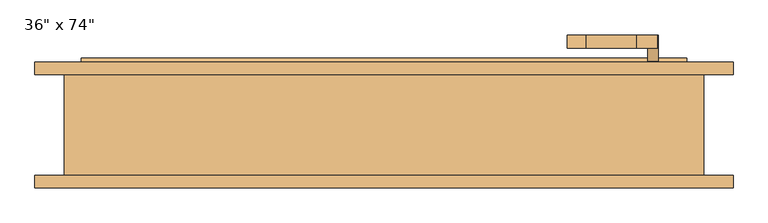
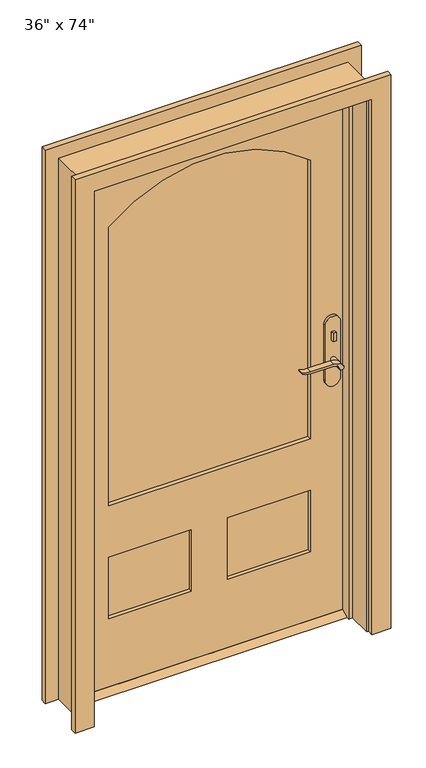
"""IFC4 building model written with IfcOpenShell, lengths in millimetres: door geometry."""

from ifc_helpers import new_model, si_unit, point, frame, frame_2d, origin, place, context, project, spatial, polyline, circle_curve, trimmed, segment, composite_curve, outline, extrude, faceted_brep, source, transform, mapped, element, save


def door_6e7732ad(model_context):
    return source(origin(), model_context, "Body", "SolidModel", [
        extrude(outline(polyline([(38.1, 12.7), (73.025, 12.7), (98.425, 0.0), (12.7, 0.0), (38.1, 12.7)])), frame((-457.2, 0.0, 0.0), z_axis=(1.0, 0.0, 0.0), x_axis=(0.0, 1.0, 0.0)), (0.0, 0.0, 1.0), 914.4),
        extrude(outline(polyline([(411.4, 18.1), (401.4, 18.1), (401.4, 28.1), (411.4, 28.1), (411.4, 18.1)])), frame((0.0, 0.0, 981.9), z_axis=(0.0, 0.0, 1.0), x_axis=(1.0, 0.0, 0.0)), (0.0, 0.0, 1.0), 30.0),
        extrude(outline(composite_curve([segment(trimmed(circle_curve(frame_2d((996.9, 406.4)), 8.0), [point((996.9, 398.4))], [point((996.9, 414.4))], False, "CARTESIAN"), True, "CONTINUOUS"), segment(trimmed(circle_curve(frame_2d((996.9, 406.4)), 8.0), [point((996.9, 414.4))], [point((996.9, 398.4))], False, "CARTESIAN"), True, "CONTINUOUS")], self_intersect=False)), frame((0.0, 83.025, 0.0), z_axis=(0.0, 1.0, 0.0), x_axis=(0.0, 0.0, 1.0)), (0.0, 0.0, 1.0), 10.0),
        extrude(outline(composite_curve([segment(trimmed(circle_curve(frame_2d((897.1555521, 382.7324871)), 37.2832219), [point((919.0523287, 412.9081363))], [point((934.4, 381.0325667))], False, "CARTESIAN"), True, "CONTINUOUS"), segment(polyline([(934.4, 381.0325667), (934.4, 304.7564091)]), True, "CONTINUOUS"), segment(trimmed(circle_curve(frame_2d((1017.6850638, 304.8227909)), 83.2850902), [point((934.4, 304.7564091))], [point((939.4, 276.4))], True, "CARTESIAN"), True, "CONTINUOUS"), segment(polyline([(939.4, 276.4), (936.6135558, 276.4)]), True, "CONTINUOUS"), segment(trimmed(circle_curve(frame_2d((986.6709207, 308.3396612)), 59.3791355), [point((936.6135558, 276.4))], [point((927.4, 304.7564091))], False, "CARTESIAN"), True, "CONTINUOUS"), segment(polyline([(927.4, 304.7564091), (927.4, 381.0138099)]), True, "CONTINUOUS"), segment(trimmed(circle_curve(frame_2d((909.2738613, 381.0138099)), 18.1261387), [point((927.4, 381.0138099))], [point((914.4, 398.4))], True, "CARTESIAN"), True, "CONTINUOUS"), segment(trimmed(circle_curve(frame_2d((914.4, 406.4)), 8.0), [point((914.4, 398.4))], [point((919.0523287, 412.9081363))], False, "CARTESIAN"), True, "CONTINUOUS")], self_intersect=False)), frame((0.0, -21.9, 0.0), z_axis=(0.0, 1.0, 0.0), x_axis=(0.0, 0.0, 1.0)), (0.0, 0.0, 1.0), 20.0),
        extrude(outline(composite_curve([segment(trimmed(circle_curve(frame_2d((914.4, 406.4)), 8.0), [point((914.3999903, 398.4))], [point((919.0523287, 412.9081363))], False, "CARTESIAN"), True, "CONTINUOUS"), segment(trimmed(circle_curve(frame_2d((897.1555521, 382.7324871)), 37.2832219), [point((919.0523287, 412.9081363))], [point((934.4, 381.0325667))], False, "CARTESIAN"), True, "CONTINUOUS"), segment(polyline([(934.4, 381.0325667), (934.4, 304.7564091)]), True, "CONTINUOUS"), segment(trimmed(circle_curve(frame_2d((1017.6850638, 304.8227909)), 83.2850902), [point((934.4, 304.7564091))], [point((939.4, 276.4))], True, "CARTESIAN"), True, "CONTINUOUS"), segment(polyline([(939.4, 276.4), (936.6135558, 276.4)]), True, "CONTINUOUS"), segment(trimmed(circle_curve(frame_2d((986.6709207, 308.3396612)), 59.3791355), [point((936.6135558, 276.4))], [point((927.4, 304.7564091))], False, "CARTESIAN"), True, "CONTINUOUS"), segment(polyline([(927.4, 304.7564091), (927.4, 381.0138122)]), True, "CONTINUOUS"), segment(trimmed(circle_curve(frame_2d((909.2738682, 381.0138122)), 18.1261318), [point((927.4, 381.0138122))], [point((914.3999903, 398.4))], True, "CARTESIAN"), True, "CONTINUOUS")], self_intersect=False)), frame((0.0, 113.025, 0.0), z_axis=(0.0, 1.0, 0.0), x_axis=(0.0, 0.0, 1.0)), (0.0, 0.0, 1.0), 20.0),
        extrude(outline(composite_curve([segment(trimmed(circle_curve(frame_2d((914.4, 406.4)), 8.0), [point((914.4, 398.4))], [point((914.4, 414.4))], False, "CARTESIAN"), True, "CONTINUOUS"), segment(trimmed(circle_curve(frame_2d((914.4, 406.4)), 8.0), [point((914.4, 414.4))], [point((914.4, 398.4))], False, "CARTESIAN"), True, "CONTINUOUS")], self_intersect=False)), frame((0.0, -1.9, 0.0), z_axis=(0.0, 1.0, 0.0), x_axis=(0.0, 0.0, 1.0)), (0.0, 0.0, 1.0), 30.0),
        extrude(outline(composite_curve([segment(trimmed(circle_curve(frame_2d((914.4, 406.4)), 8.0), [point((914.4, 398.4))], [point((914.4, 414.4))], False, "CARTESIAN"), True, "CONTINUOUS"), segment(trimmed(circle_curve(frame_2d((914.4, 406.4)), 8.0), [point((914.4, 414.4))], [point((914.4, 398.4))], False, "CARTESIAN"), True, "CONTINUOUS")], self_intersect=False)), frame((0.0, 83.025, 0.0), z_axis=(0.0, 1.0, 0.0), x_axis=(0.0, 0.0, 1.0)), (0.0, 0.0, 1.0), 30.0),
        extrude(outline(composite_curve([segment(polyline([(844.4, 431.4), (1039.4, 431.4)]), True, "CONTINUOUS"), segment(trimmed(circle_curve(frame_2d((1039.4, 406.4)), 25.0), [point((1039.4, 431.4))], [point((1039.4, 381.4))], False, "CARTESIAN"), True, "CONTINUOUS"), segment(polyline([(1039.4, 381.4), (844.4, 381.4)]), True, "CONTINUOUS"), segment(trimmed(circle_curve(frame_2d((844.4, 406.4)), 25.0), [point((844.4, 381.4))], [point((844.4, 431.4))], False, "CARTESIAN"), True, "CONTINUOUS")], self_intersect=False)), frame((0.0, 28.1, 0.0), z_axis=(0.0, 1.0, 0.0), x_axis=(0.0, 0.0, 1.0)), (0.0, 0.0, 1.0), 10.0),
        extrude(outline(composite_curve([segment(polyline([(844.4, 431.4), (1039.4, 431.4)]), True, "CONTINUOUS"), segment(trimmed(circle_curve(frame_2d((1039.4, 406.4)), 25.0), [point((1039.4, 431.4))], [point((1039.4, 381.4))], False, "CARTESIAN"), True, "CONTINUOUS"), segment(polyline([(1039.4, 381.4), (844.4, 381.4)]), True, "CONTINUOUS"), segment(trimmed(circle_curve(frame_2d((844.4, 406.4)), 25.0), [point((844.4, 381.4))], [point((844.4, 431.4))], False, "CARTESIAN"), True, "CONTINUOUS")], self_intersect=False)), frame((0.0, 73.025, 0.0), z_axis=(0.0, 1.0, 0.0), x_axis=(0.0, 0.0, 1.0)), (0.0, 0.0, 1.0), 10.0),
        extrude(outline(polyline([(1879.6, -457.2), (12.7, -457.2), (12.7, 457.2), (1879.6, 457.2), (1879.6, -457.2)]), holes=[composite_curve([segment(polyline([(650.875, -336.55), (1631.95, -336.55)]), True, "CONTINUOUS"), segment(trimmed(circle_curve(frame_2d((1249.52125, 0.0)), 509.42875), [point((1631.95, -336.55))], [point((1631.95, 336.55))], True, "CARTESIAN"), True, "CONTINUOUS"), segment(polyline([(1631.95, 336.55), (650.875, 336.55), (650.875, -336.55)]), True, "CONTINUOUS")], self_intersect=False), polyline([(469.9, -60.325), (254.0, -60.325), (254.0, -336.55), (469.9, -336.55), (469.9, -60.325)]), polyline([(469.9, 336.55), (254.0, 336.55), (254.0, 60.325), (469.9, 60.325), (469.9, 336.55)])]), frame((0.0, 38.1, 0.0), z_axis=(0.0, 1.0, 0.0), x_axis=(0.0, 0.0, 1.0)), (0.0, 0.0, 1.0), 34.925),
        faceted_brep([(482.6, 73.025, 0.0), (482.6, -79.375, 0.0), (457.2, -79.375, 0.0), (457.2, 3.175, 0.0), (444.5, 3.175, 0.0), (444.5, 38.1, 0.0), (457.2, 38.1, 0.0), (457.2, 73.025, 0.0), (482.6, 73.025, 1905.0), (482.6, -79.375, 1905.0), (-482.6, -79.375, 1905.0), (-482.6, -79.375, 0.0), (-457.2, -79.375, 0.0), (-457.2, -79.375, 1879.6), (457.2, -79.375, 1879.6), (457.2, 3.175, 1879.6), (-457.2, 3.175, 1879.6), (-457.2, 3.175, 0.0), (-444.5, 3.175, 0.0), (-444.5, 3.175, 1866.9), (444.5, 3.175, 1866.9), (444.5, 38.1, 1866.9), (-444.5, 38.1, 1866.9), (-444.5, 38.1, 0.0), (-457.2, 38.1, 0.0), (-457.2, 38.1, 1879.6), (457.2, 38.1, 1879.6), (457.2, 73.025, 1879.6), (-457.2, 73.025, 1879.6), (-457.2, 73.025, 0.0), (-482.6, 73.025, 0.0), (-482.6, 73.025, 1905.0)], [[[0, 1, 2, 3, 4, 5, 6, 7]], [[1, 0, 8, 9]], [[2, 1, 9, 10, 11, 12, 13, 14]], [[3, 2, 14, 15]], [[4, 3, 15, 16, 17, 18, 19, 20]], [[5, 4, 20, 21]], [[6, 5, 21, 22, 23, 24, 25, 26]], [[7, 6, 26, 27]], [[0, 7, 27, 28, 29, 30, 31, 8]], [[9, 8, 31, 10]], [[15, 14, 13, 16]], [[21, 20, 19, 22]], [[27, 26, 25, 28]], [[30, 29, 24, 23, 18, 17, 12, 11]], [[10, 31, 30, 11]], [[16, 13, 12, 17]], [[22, 19, 18, 23]], [[28, 25, 24, 29]]]),
        extrude(outline(polyline([(-60.325, 49.7416667), (-336.55, 49.7416667), (-336.55, 61.3833333), (-60.325, 61.3833333), (-60.325, 49.7416667)])), frame((0.0, 0.0, 254.0), z_axis=(0.0, 0.0, 1.0), x_axis=(1.0, 0.0, 0.0)), (0.0, 0.0, 1.0), 215.9),
        extrude(outline(polyline([(336.55, 49.7416667), (60.325, 49.7416667), (60.325, 61.3833333), (336.55, 61.3833333), (336.55, 49.7416667)])), frame((0.0, 0.0, 254.0), z_axis=(0.0, 0.0, 1.0), x_axis=(1.0, 0.0, 0.0)), (0.0, 0.0, 1.0), 215.9),
        extrude(outline(composite_curve([segment(polyline([(650.875, -336.55), (650.875, 336.55), (1631.95, 336.55)]), True, "CONTINUOUS"), segment(trimmed(circle_curve(frame_2d((1249.52125, 0.0)), 509.42875), [point((1631.95, 336.55))], [point((1631.95, -336.55))], False, "CARTESIAN"), True, "CONTINUOUS"), segment(polyline([(1631.95, -336.55), (650.875, -336.55)]), True, "CONTINUOUS")], self_intersect=False)), frame((0.0, 52.07, 0.0), z_axis=(0.0, 1.0, 0.0), x_axis=(0.0, 0.0, 1.0)), (0.0, 0.0, 1.0), 6.985),
        extrude(outline(polyline([(0.0, -527.05), (0.0, -463.55), (1885.95, -463.55), (1885.95, 463.55), (0.0, 463.55), (0.0, 527.05), (1949.45, 527.05), (1949.45, -527.05), (0.0, -527.05)])), frame((0.0, -98.425, 0.0), z_axis=(0.0, 1.0, 0.0), x_axis=(0.0, 0.0, 1.0)), (0.0, 0.0, 1.0), 19.05),
        extrude(outline(polyline([(0.0, -527.05), (0.0, -463.55), (1885.95, -463.55), (1885.95, 463.55), (0.0, 463.55), (0.0, 527.05), (1949.45, 527.05), (1949.45, -527.05), (0.0, -527.05)])), frame((0.0, 73.025, 0.0), z_axis=(0.0, 1.0, 0.0), x_axis=(0.0, 0.0, 1.0)), (0.0, 0.0, 1.0), 19.05),
    ])


if __name__ == "__main__":
    model = new_model("IFC4")
    model_context = context("Model", 3, world=origin())
    ifc_project = project(units=[si_unit("LENGTHUNIT", "METRE", prefix="MILLI")], contexts=[model_context])
    site = spatial("IfcSite", under=ifc_project)
    building = spatial("IfcBuilding", under=site)
    placement = place(None, origin())
    door_shape = door_6e7732ad(model_context)
    element("IfcDoor", 1, ObjectType="36\" x 74\"", at=placement, inside=building, context=model_context, shape_type="MappedRepresentation", body=[
        mapped(door_shape, transform((0.0, 0.0, 0.0), x_axis=(1.0, 0.0, 0.0), y_axis=(0.0, 1.0, 0.0), z_axis=(0.0, 0.0, 1.0))),
    ])
    save(model, "model.ifc")

# Revit data of these elements
# Type "36\" x 74\""
#   Type Mark = "8"
#   Assembly Code = "B2030100"
#   Analytic Construction = "French door, wood frame with single glass"
#   Threshold Offset [instance default] = 0' - 0 1/2"
#   Thickness = 0' - 1 3/8"
#   Thermal Resistance (R) = 1.0696 (h·ft²·°F)/BTU
#   Swing Angle [instance default] = 90.00°
#   Stiles = 0' - 4 3/4"
#   Rough Width = 3' - 2"
#   Rough Height = 6' - 3"
#   Radius = 1' - 8.05625"
#   Lock Rail = 0' - 7 1/8"
#   Height = 6' - 2"
#   Width = 3' - 0"
#   Heat Transfer Coefficient (U) = 0.9350 BTU/(h·ft²·°F)
#   Door Offset [instance default] = 0' - 0"
#   Bottom Rail = 0' - 9 1/2"
#   Threshold [instance default] = yes
#   Function = 1
#   Exterior Trim [instance default] = yes
#   Trim Material = Cherry
#   Threshold Material = Cherry
#   Panel Material = Cherry
#   Glazing = Glass
#   Frame Material = Cherry
#   Door Handle Material = Aluminum
#   Visual Light Transmittance = 0
#   Solar Heat Gain Coefficient = 0
#   Wall Closure = (empty or 0)
#   Construction Type = (empty or 0)
# Element 1 (IfcDoor, "36\" x 74\"")
#   Materials on its faces: "Cherry", "Aluminum", "Glass"
# Materials
#   "Cherry": class "Wood", colour RGB 226 177 128, transparency 0, Description = "Prunus Serotina", Cost = 0
#   "Glass": class "Glass", colour RGB 0 128 192, transparency 0.75, Description = "Soda Lime Glass", Cost = 0
#   "Aluminum": class "Metal", colour RGB 247 247 247, transparency 0, Description = "Aluminum 6061", Cost = 0
